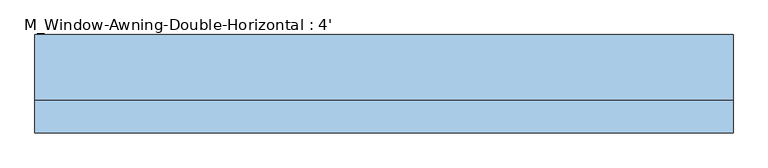
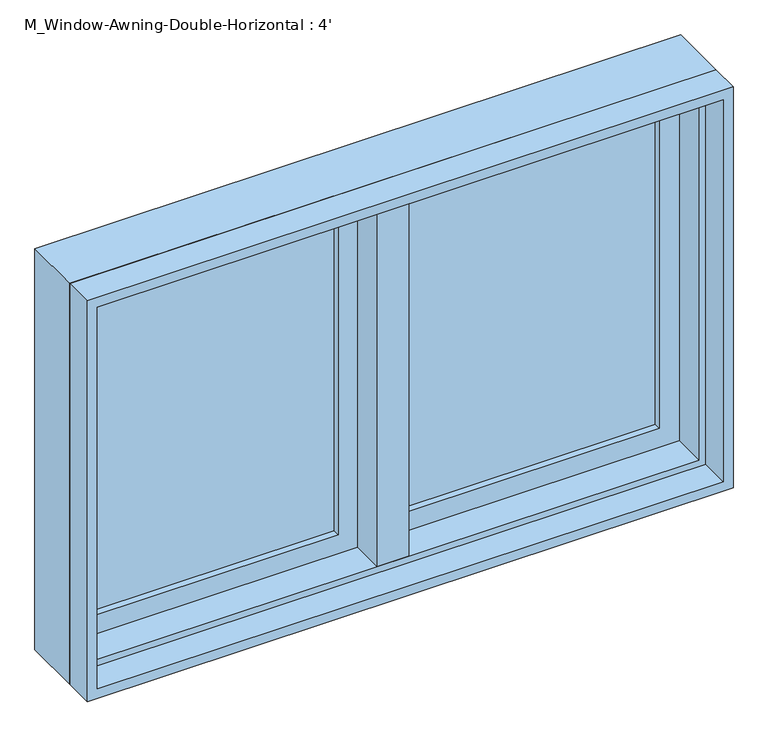
"""IFC4 building model written with IfcOpenShell, lengths in millimetres: window geometry, M_Window-Awning-Double-Horizontal : 4'."""

from ifc_helpers import new_model, si_unit, frame, origin, place, context, project, spatial, polyline, outline, extrude, faceted_brep, source, transform, mapped, element, save


def m_window_awning_double_horizontal_4_cab21571(model_context):
    return source(origin(), model_context, "Body", "SolidModel", [
        faceted_brep([(577.85, 44.45, 1668.25), (577.85, -19.05, 1668.25), (-577.85, -19.05, 1668.25), (-577.85, 44.45, 1668.25), (596.9, 95.25, 1687.3), (596.9, 44.45, 1687.3), (-596.9, 44.45, 1687.3), (-596.9, 95.25, 1687.3), (609.6, -19.05, 1700.0), (609.6, 95.25, 1700.0), (-609.6, 95.25, 1700.0), (-609.6, -19.05, 1700.0), (-577.85, -19.05, 931.75), (-577.85, 44.45, 931.75), (-596.9, 44.45, 912.7), (-596.9, 95.25, 912.7), (-609.6, 95.25, 900.0), (-609.6, -19.05, 900.0), (577.85, -19.05, 931.75), (577.85, 44.45, 931.75), (596.9, 44.45, 912.7), (596.9, 95.25, 912.7), (609.6, 95.25, 900.0), (609.6, -19.05, 900.0)], [[[0, 1, 2, 3]], [[4, 5, 6, 7]], [[8, 9, 10, 11]], [[3, 2, 12, 13]], [[7, 6, 14, 15]], [[11, 10, 16, 17]], [[13, 12, 18, 19]], [[15, 14, 20, 21]], [[17, 16, 22, 23]], [[11, 17, 23, 8], [1, 18, 12, 2]], [[19, 18, 1, 0]], [[5, 20, 14, 6], [3, 13, 19, 0]], [[21, 20, 5, 4]], [[23, 22, 9, 8]], [[9, 22, 16, 10], [7, 15, 21, 4]]]),
        extrude(outline(polyline([(1700.0, -609.6), (900.0, -609.6), (900.0, 609.6), (1700.0, 609.6), (1700.0, -609.6)]), holes=[polyline([(1680.95, 590.55), (919.05, 590.55), (919.05, -590.55), (1680.95, -590.55), (1680.95, 590.55)])]), frame((0.0, -76.2, 0.0), z_axis=(0.0, 1.0, 0.0), x_axis=(0.0, 0.0, 1.0)), (0.0, 0.0, 1.0), 57.15),
        extrude(outline(polyline([(912.7, 596.9), (1687.3, 596.9), (1687.3, 9.525), (912.7, 9.525), (912.7, 596.9)]), holes=[polyline([(969.85, 66.675), (1630.15, 66.675), (1630.15, 539.75), (969.85, 539.75), (969.85, 66.675)])]), frame((0.0, 44.45, 0.0), z_axis=(0.0, 1.0, 0.0), x_axis=(0.0, 0.0, 1.0)), (0.0, 0.0, 1.0), 44.45),
        extrude(outline(polyline([(1687.3, -596.9), (912.7, -596.9), (912.7, -9.525), (1687.3, -9.525), (1687.3, -596.9)]), holes=[polyline([(1630.15, -66.675), (969.85, -66.675), (969.85, -539.75), (1630.15, -539.75), (1630.15, -66.675)])]), frame((0.0, 44.45, 0.0), z_axis=(0.0, 1.0, 0.0), x_axis=(0.0, 0.0, 1.0)), (0.0, 0.0, 1.0), 44.45),
        extrude(outline(polyline([(539.75, 76.2), (539.75, 69.85), (66.675, 69.85), (66.675, 76.2), (539.75, 76.2)])), frame((0.0, 0.0, 969.85), z_axis=(0.0, 0.0, 1.0), x_axis=(1.0, 0.0, 0.0)), (0.0, 0.0, 1.0), 660.3),
        extrude(outline(polyline([(66.675, 57.15), (66.675, 63.5), (539.75, 63.5), (539.75, 57.15), (66.675, 57.15)])), frame((0.0, 0.0, 969.85), z_axis=(0.0, 0.0, 1.0), x_axis=(1.0, 0.0, 0.0)), (0.0, 0.0, 1.0), 660.3),
        extrude(outline(polyline([(-66.675, 76.2), (-66.675, 69.85), (-539.75, 69.85), (-539.75, 76.2), (-66.675, 76.2)])), frame((0.0, 0.0, 969.85), z_axis=(0.0, 0.0, 1.0), x_axis=(1.0, 0.0, 0.0)), (0.0, 0.0, 1.0), 660.3),
        extrude(outline(polyline([(-539.75, 57.15), (-539.75, 63.5), (-66.675, 63.5), (-66.675, 57.15), (-539.75, 57.15)])), frame((0.0, 0.0, 969.85), z_axis=(0.0, 0.0, 1.0), x_axis=(1.0, 0.0, 0.0)), (0.0, 0.0, 1.0), 660.3),
        faceted_brep([(9.525, 95.25, 1687.3), (-9.525, 95.25, 1687.3), (-9.525, 44.45, 1687.3), (9.525, 44.45, 1687.3), (9.525, 95.25, 912.7), (9.525, 44.45, 912.7), (-9.525, 44.45, 912.7), (-9.525, 95.25, 912.7), (-9.525, 44.45, 931.75), (-9.525, 44.45, 1668.25), (-30.1625, 44.45, 931.75), (-30.1625, 44.45, 1668.25), (-30.1625, -19.05, 931.75), (-30.1625, -19.05, 1668.25), (30.1625, -19.05, 931.75), (30.1625, -19.05, 1668.25), (30.1625, 44.45, 931.75), (30.1625, 44.45, 1668.25), (9.525, 44.45, 931.75), (9.525, 44.45, 1668.25)], [[[0, 1, 2, 3]], [[4, 5, 6, 7]], [[1, 0, 4, 7]], [[2, 1, 7, 6, 8, 9]], [[9, 8, 10, 11]], [[11, 10, 12, 13]], [[13, 12, 14, 15]], [[15, 14, 16, 17]], [[17, 16, 18, 19]], [[0, 3, 19, 18, 5, 4]], [[18, 8, 6, 5]], [[9, 19, 3, 2]], [[8, 18, 16, 14, 12, 10]], [[19, 9, 11, 13, 15, 17]]]),
    ])


if __name__ == "__main__":
    model = new_model("IFC4")
    model_context = context("Model", 3, world=origin())
    ifc_project = project(units=[si_unit("LENGTHUNIT", "METRE", prefix="MILLI")], contexts=[model_context])
    site = spatial("IfcSite", under=ifc_project)
    building = spatial("IfcBuilding", under=site)
    placement = place(None, origin())
    m_window_awning_double_horizontal_4_shape = m_window_awning_double_horizontal_4_cab21571(model_context)
    element("IfcWindow", 1, ObjectType="M_Window-Awning-Double-Horizontal : 4'", at=placement, inside=building, context=model_context, shape_type="MappedRepresentation", body=[
        mapped(m_window_awning_double_horizontal_4_shape, transform((0.0, 0.0, 0.0), x_axis=(1.0, 0.0, 0.0), y_axis=(0.0, 1.0, 0.0), z_axis=(0.0, 0.0, 1.0))),
    ])
    save(model, "model.ifc")

# Revit data of these elements
# Type "M_Window-Awning-Double-Horizontal : 4'"
#   Type Mark = "28"
#   Fire Rating = "0.5h"
#   Assembly Code = "B2020100"
#   Analytic Construction = "Double glazing - domestic"
#   Window Inset [instance default] = 0' - 0"
#   Wall Thickness [instance default] = 0' - 5.90551"
#   Interior Wall Closure [instance default] = 0' - 2.15551"
#   Half Width = 2' - 0"
#   Visual Light Transmittance = 0.81
#   Thermal Resistance (R) = 0.319569 (m²·K)/W
#   Solar Heat Gain Coefficient = 0.76
#   Rough Width = 4' - 0.59055"
#   Rough Height = 2' - 8.08661"
#   Height = 2' - 7.49606"
#   Heat Transfer Coefficient (U) = 3.12929 W/(m²·K)
#   Frame Extension [instance default] = 0' - 0 1/4"
#   Exterior Wall Closure [instance default] = 0' - 1 1/4"
#   Extension Jamb [instance default] = 0' - 2.15551"
#   Default Sill Height = 2' - 11.43307"
#   Width = 4' - 0"
#   Muntin Visibility = yes
#   Interior Trim Visibility [instance default] = yes
#   Exterior Trim Visibility [instance default] = yes
#   Extension Jamb Visibility [instance default] = yes
#   Interior Trim Material = Wood - Stained
#   Muntin Pattern = M_Muntin Pattern_2x2 : M_Muntin Pattern_2x2
#   Interior Trim = M_Trim-Window-Interior-Flat : Picture Frame
#   Interior Frame Material = Wood - Stained
#   Glass Panel Material = Glass
#   Exterior Trim Material = Clad - White
#   Exterior Trim = M_Trim-Window-Exterior-Flat : with Sill
#   Exterior Frame Material = Clad - White
#   Wall Closure = (empty or 0)
# Element 1 (IfcWindow, "M_Window-Awning-Double-Horizontal : 4'")
#   Wall Thickness = 0' - 6"
#   Extension Jamb = 0' - 2 1/4"
#   Materials on its faces: "Wood - Stained", "Glass", "Clad - White"
# Materials
#   "Wood - Stained": class "Wood", colour RGB 224 178 126, transparency 0, Cost = 0
#   "Glass": class "Glass", colour RGB 0 128 192, transparency 0.9, Description = "Soda Lime Glass", Cost = 0
#   "Clad - White": class "Wood", colour RGB 242 242 238, transparency 0, Cost = 0
